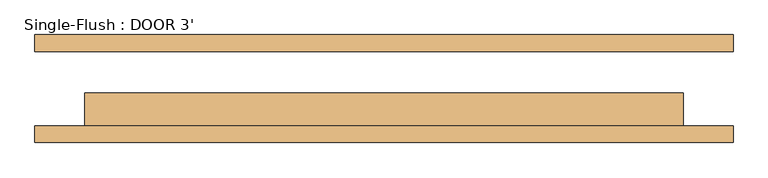
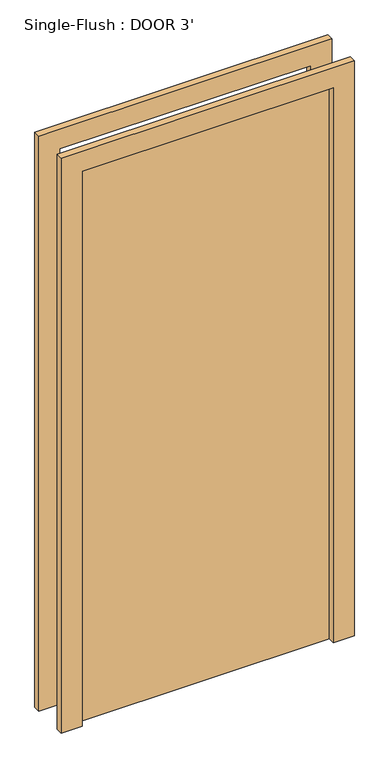
"""IFC4 building model written with IfcOpenShell, lengths in millimetres: door geometry, Single-Flush : DOOR 3'."""

from ifc_helpers import new_model, si_unit, frame, origin, origin_with_axes, place, context, project, spatial, polyline, outline, extrude, source, transform, mapped, element, save


def single_flush_door_3_305aa2a5(model_context):
    return source(origin(), model_context, "Body", "SweptSolid", [
        extrude(outline(polyline([(2209.8, -533.4), (0.0, -533.4), (0.0, -457.2), (2133.6, -457.2), (2133.6, 457.2), (0.0, 457.2), (0.0, 533.4), (2209.8, 533.4), (2209.8, -533.4)])), frame((0.0, -82.55, 0.0), z_axis=(0.0, 1.0, 0.0), x_axis=(0.0, 0.0, 1.0)), (0.0, 0.0, 1.0), 25.4),
        extrude(outline(polyline([(2209.8, 533.4), (2209.8, -533.4), (0.0, -533.4), (0.0, -457.2), (2133.6, -457.2), (2133.6, 457.2), (0.0, 457.2), (0.0, 533.4), (2209.8, 533.4)])), frame((0.0, 57.15, 0.0), z_axis=(0.0, 1.0, 0.0), x_axis=(0.0, 0.0, 1.0)), (0.0, 0.0, 1.0), 25.4),
        extrude(outline(polyline([(457.2, -6.35), (457.2, -57.15), (-457.2, -57.15), (-457.2, -6.35), (457.2, -6.35)])), origin_with_axes(), (0.0, 0.0, 1.0), 2133.6),
    ])


if __name__ == "__main__":
    model = new_model("IFC4")
    model_context = context("Model", 3, world=origin())
    ifc_project = project(units=[si_unit("LENGTHUNIT", "METRE", prefix="MILLI")], contexts=[model_context])
    site = spatial("IfcSite", under=ifc_project)
    building = spatial("IfcBuilding", under=site)
    placement = place(None, origin())
    single_flush_door_3_shape = single_flush_door_3_305aa2a5(model_context)
    element("IfcDoor", 1, ObjectType="Single-Flush : DOOR 3'", at=placement, inside=building, context=model_context, shape_type="MappedRepresentation", body=[
        mapped(single_flush_door_3_shape, transform((0.0, 0.0, 0.0), x_axis=(1.0, 0.0, 0.0), y_axis=(0.0, 1.0, 0.0), z_axis=(0.0, 0.0, 1.0))),
    ])
    save(model, "model.ifc")

# Revit data of these elements
# Type "Single-Flush : DOOR 3'"
#   Type Mark = "8"
#   Construction Type Id = "MDOOR"
#   Assembly Code = "C1020"
#   Analytic Construction = "Metal"
#   Thickness = 0' - 2"
#   Heat Transfer Coefficient (U) = 0.651978 BTU/(h·ft²·°F)
#   Height = 7' - 0"
#   Trim Projection Ext = 0' - 1"
#   Trim Projection Int = 0' - 1"
#   Trim Width = 0' - 3"
#   Width = 3' - 0"
#   Define Thermal Properties by = 1
#   Door Material = Door - Panel
#   Frame Material = Door - Frame
#   Visual Light Transmittance = 0
#   Solar Heat Gain Coefficient = 0
#   Function = (empty or 0)
#   Wall Closure = (empty or 0)
# Element 1 (IfcDoor, "Single-Flush : DOOR 3'")
#   Materials on its faces: "Door - Frame", "Door - Panel"
# Materials
#   "Door - Panel": class "Wood", colour RGB 210 159 95, transparency 0, Cost = 0
#   "Door - Frame": colour RGB 118 70 51, transparency 0, Cost = 0
